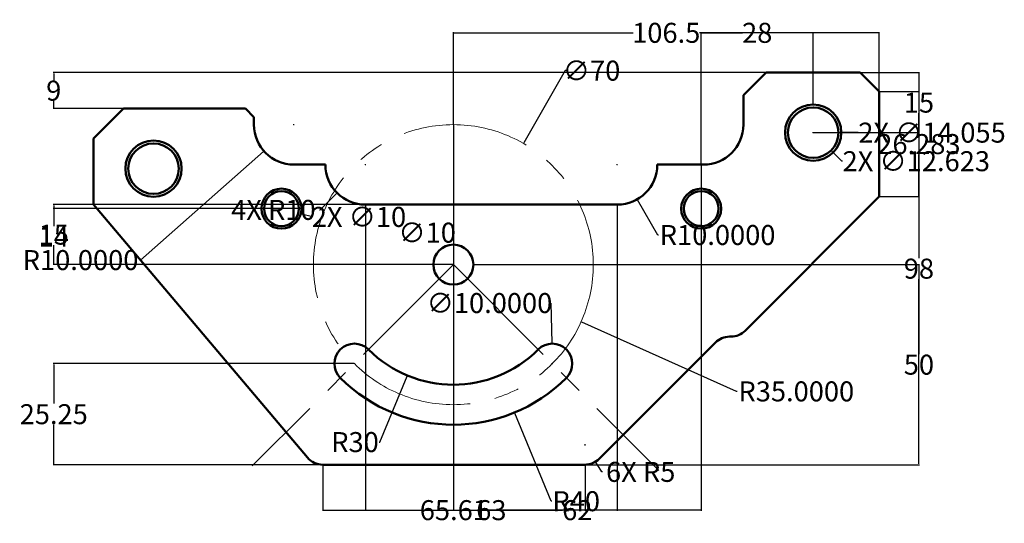
# Model space of a CAD drawing. Units: inches. Extents: x 2702 to 2948, y 1752 to 1878.
import ezdxf

# ---------------------------------------------------------------- set-up
doc = ezdxf.new("R2010")
doc.units = ezdxf.units.IN
doc.header["$MEASUREMENT"] = 0
doc.linetypes.add('CENTER', pattern=[50.8, 31.75, -6.35, 6.35, -6.35])
for name, color, linetype, lineweight in [('M-CNTR', 4, 'CENTER', 18), ('M-CONS', 8, 'Continuous', 13), ('M-DIMS', 2, 'Continuous', 25), ('M-OUTL', 7, 'Continuous', 50)]:
    doc.layers.add(name, color=color, linetype=linetype, lineweight=lineweight)
doc.styles.get("Standard").update_dxf_attribs({"font": 'arial.ttf'})
doc.dimstyles.get("Standard").update_dxf_attribs({"dimtxt": 5, "dimasz": 0.18, "dimexe": 0.18, "dimexo": 0.0625, "dimgap": 0.09, "dimtad": 0, "dimtih": 1, "dimtoh": 1, "dimdec": 4, "dimzin": 0, "dimdsep": 46, "dimtxsty": 'Standard', "dimcen": 0.09, "dimadec": 0, "dimazin": 0, "dimtfac": 1, "dimtdec": 4, "dimtofl": 0, "dimtmove": 0, "dimatfit": 3, "dimfxl": 1, "dimtolj": 1, "dimtzin": 0, "dimarcsym": 0})

# ---------------------------------------------------------------- blocks, each defined once
blk = doc.blocks.new('*D1')
at = {"layer": 'Defpoints', "color": 0, "transparency": 16777216}
for p in [(2851.5, 1841.74), (2856.48, 1833.07)]:
    blk.add_point(p, dxfattribs=at)
at = {"layer": 'M-DIMS', "color": 0, "lineweight": -2, "transparency": 16777216}
for p, q in [((2851.41, 1841.74), (2851.59, 1841.74)), ((2851.5, 1841.65), (2851.5, 1841.83)), ((2861.61, 1824.15), (2856.57, 1832.91)), ((2861.79, 1824.15), (2861.61, 1824.15))]:
    blk.add_line(p, q, dxfattribs=at)
at = {"layer": 'M-DIMS', "color": 0, "transparency": 16777216}
blk.add_solid([(2856.6, 1832.93), (2856.55, 1832.9), (2856.48, 1833.07)], dxfattribs=at)
at = {"layer": 'M-DIMS', "color": 0, "transparency": 16777216, "insert": (2876.59, 1824.15), "char_height": 5, "attachment_point": 5}
blk.add_mtext('\\A1;R10.0000', dxfattribs=at)
blk = doc.blocks.new('*D2')
at = {"layer": 'Defpoints', "color": 0, "transparency": 16777216}
for p in [(2770.62, 1851.74), (2763.12, 1845.12)]:
    blk.add_point(p, dxfattribs=at)
at = {"layer": 'M-DIMS', "color": 0, "lineweight": -2, "transparency": 16777216}
for p, q in [((2770.53, 1851.74), (2770.71, 1851.74)), ((2770.62, 1851.65), (2770.62, 1851.83)), ((2732.22, 1817.88), (2762.98, 1845.01)), ((2732.04, 1817.88), (2732.22, 1817.88))]:
    blk.add_line(p, q, dxfattribs=at)
at = {"layer": 'M-DIMS', "color": 0, "transparency": 16777216}
blk.add_solid([(2762.97, 1845.03), (2763, 1844.98), (2763.12, 1845.12)], dxfattribs=at)
at = {"layer": 'M-DIMS', "color": 0, "transparency": 16777216, "insert": (2717.25, 1817.88), "char_height": 5, "attachment_point": 5}
blk.add_mtext('\\A1;R10.0000', dxfattribs=at)
blk = doc.blocks.new('*D3')
at = {"layer": 'Defpoints', "color": 0, "transparency": 16777216}
for p in [(2810.5, 1816.74), (2842.45, 1802.45)]:
    blk.add_point(p, dxfattribs=at)
at = {"layer": 'M-DIMS', "color": 0, "lineweight": -2, "transparency": 16777216}
for p, q in [((2810.41, 1816.74), (2810.59, 1816.74)), ((2810.5, 1816.65), (2810.5, 1816.83)), ((2881.3, 1785.06), (2842.61, 1802.37)), ((2881.48, 1785.06), (2881.3, 1785.06))]:
    blk.add_line(p, q, dxfattribs=at)
at = {"layer": 'M-DIMS', "color": 0, "transparency": 16777216}
blk.add_solid([(2842.62, 1802.4), (2842.6, 1802.34), (2842.45, 1802.45)], dxfattribs=at)
at = {"layer": 'M-DIMS', "color": 0, "transparency": 16777216, "insert": (2896.28, 1785.06), "char_height": 5, "attachment_point": 5}
blk.add_mtext('\\A1;R35.0000', dxfattribs=at)
blk = doc.blocks.new('*D4')
at = {"layer": 'Defpoints', "color": 0, "transparency": 16777216}
for p in [(2835.11, 1796.99), (2835.38, 1786.99)]:
    blk.add_point(p, dxfattribs=at)
at = {"layer": 'M-DIMS', "color": 0, "lineweight": -2, "transparency": 16777216}
for p, q in [((2834.66, 1807.14), (2834.84, 1807.14)), ((2834.84, 1807.14), (2835.11, 1797.17)), ((2835.16, 1791.99), (2835.34, 1791.99)), ((2835.25, 1791.9), (2835.25, 1792.08))]:
    blk.add_line(p, q, dxfattribs=at)
at = {"layer": 'M-DIMS', "color": 0, "transparency": 16777216}
blk.add_solid([(2835.14, 1797.17), (2835.08, 1797.17), (2835.11, 1796.99)], dxfattribs=at)
at = {"layer": 'M-DIMS', "color": 0, "transparency": 16777216, "insert": (2819.53, 1807.14), "char_height": 5, "attachment_point": 5}
blk.add_mtext('\\A1;∅10.0000', dxfattribs=at)
blk = doc.blocks.new('MOUNT-HOLE-LARGE')
for radius in [7.03, 7.03, 7.03, 6.31]:
    blk.add_circle((0, 0), radius)
blk = doc.blocks.new('MOUNT-HOLE-SMALL')
for radius in [5, 4.36]:
    blk.add_circle((0, 0), radius)
blk = doc.blocks.new('*D7')
at = {"layer": 'Defpoints', "color": 0, "transparency": 16777216}
for p in [(2912.28, 1864.74), (2926.95, 1864.74), (2843.43, 1766.74)]:
    blk.add_point(p, dxfattribs=at)
at = {"layer": 'M-DIMS', "color": 0, "lineweight": -2, "transparency": 16777216}
for p, q in [((2912.35, 1864.74), (2927.13, 1864.74)), ((2926.95, 1864.56), (2926.95, 1818.38)), ((2926.95, 1766.92), (2926.95, 1813.1)), ((2843.49, 1766.74), (2927.13, 1766.74))]:
    blk.add_line(p, q, dxfattribs=at)
at = {"layer": 'M-DIMS', "color": 0, "transparency": 16777216}
for points in [[(2926.92, 1864.56), (2926.98, 1864.56), (2926.95, 1864.74)], [(2926.92, 1766.92), (2926.98, 1766.92), (2926.95, 1766.74)]]:
    blk.add_solid(points, dxfattribs=at)
at = {"layer": 'M-DIMS', "color": 0, "transparency": 16777216, "insert": (2926.95, 1815.74), "char_height": 5, "attachment_point": 5}
blk.add_mtext('\\A1;98', dxfattribs=at)
blk = doc.blocks.new('*D8')
at = {"layer": 'Defpoints', "color": 0, "transparency": 16777216}
for p in [(2917, 1874.69), (2917, 1860.02), (2810.5, 1851.74)]:
    blk.add_point(p, dxfattribs=at)
at = {"layer": 'M-DIMS', "color": 0, "lineweight": -2, "transparency": 16777216}
for p, q in [((2810.5, 1851.8), (2810.5, 1874.87)), ((2810.68, 1874.69), (2855.44, 1874.69)), ((2916.82, 1874.69), (2872.06, 1874.69)), ((2917, 1860.08), (2917, 1874.87))]:
    blk.add_line(p, q, dxfattribs=at)
at = {"layer": 'M-DIMS', "color": 0, "transparency": 16777216}
for points in [[(2810.68, 1874.72), (2810.68, 1874.66), (2810.5, 1874.69)], [(2916.82, 1874.72), (2916.82, 1874.66), (2917, 1874.69)]]:
    blk.add_solid(points, dxfattribs=at)
at = {"layer": 'M-DIMS', "color": 0, "transparency": 16777216, "insert": (2863.75, 1874.69), "char_height": 5, "attachment_point": 5}
blk.add_mtext('\\A1;106.5', dxfattribs=at)
blk = doc.blocks.new('*D9')
at = {"layer": 'Defpoints', "color": 0, "transparency": 16777216}
for p in [(2810.5, 1851.74), (2872.5, 1841.74), (2872.5, 1755.37)]:
    blk.add_point(p, dxfattribs=at)
at = {"layer": 'M-DIMS', "color": 0, "lineweight": -2, "transparency": 16777216}
for p, q in [((2810.5, 1851.68), (2810.5, 1755.19)), ((2872.5, 1841.68), (2872.5, 1755.19)), ((2810.68, 1755.37), (2837.84, 1755.37)), ((2872.32, 1755.37), (2845.16, 1755.37))]:
    blk.add_line(p, q, dxfattribs=at)
at = {"layer": 'M-DIMS', "color": 0, "transparency": 16777216}
for points in [[(2810.68, 1755.4), (2810.68, 1755.34), (2810.5, 1755.37)], [(2872.32, 1755.4), (2872.32, 1755.34), (2872.5, 1755.37)]]:
    blk.add_solid(points, dxfattribs=at)
at = {"layer": 'M-DIMS', "color": 0, "transparency": 16777216, "insert": (2841.5, 1755.37), "char_height": 5, "attachment_point": 5}
blk.add_mtext('\\A1;62', dxfattribs=at)
blk = doc.blocks.new('*D10')
at = {"layer": 'Defpoints', "color": 0, "transparency": 16777216}
for p in [(2900.5, 1874.69), (2900.5, 1856.77), (2872.5, 1841.74)]:
    blk.add_point(p, dxfattribs=at)
at = {"layer": 'M-DIMS', "color": 0, "lineweight": -2, "transparency": 16777216}
for p, q in [((2872.5, 1841.8), (2872.5, 1874.87)), ((2872.68, 1874.69), (2882.78, 1874.69)), ((2900.32, 1874.69), (2890.22, 1874.69)), ((2900.5, 1856.83), (2900.5, 1874.87))]:
    blk.add_line(p, q, dxfattribs=at)
at = {"layer": 'M-DIMS', "color": 0, "transparency": 16777216}
for points in [[(2872.68, 1874.72), (2872.68, 1874.66), (2872.5, 1874.69)], [(2900.32, 1874.72), (2900.32, 1874.66), (2900.5, 1874.69)]]:
    blk.add_solid(points, dxfattribs=at)
at = {"layer": 'M-DIMS', "color": 0, "transparency": 16777216, "insert": (2886.5, 1874.69), "char_height": 5, "attachment_point": 5}
blk.add_mtext('\\A1;28', dxfattribs=at)
blk = doc.blocks.new('*D11')
at = {"layer": 'Defpoints', "color": 0, "transparency": 16777216}
for p in [(2815.5, 1816.74), (2926.95, 1816.74), (2843.43, 1766.74)]:
    blk.add_point(p, dxfattribs=at)
at = {"layer": 'M-DIMS', "color": 0, "lineweight": -2, "transparency": 16777216}
for p, q in [((2815.56, 1816.74), (2927.13, 1816.74)), ((2926.95, 1816.56), (2926.95, 1794.38)), ((2926.95, 1766.92), (2926.95, 1789.1)), ((2843.49, 1766.74), (2927.13, 1766.74))]:
    blk.add_line(p, q, dxfattribs=at)
at = {"layer": 'M-DIMS', "color": 0, "transparency": 16777216}
for points in [[(2926.92, 1816.56), (2926.98, 1816.56), (2926.95, 1816.74)], [(2926.92, 1766.92), (2926.98, 1766.92), (2926.95, 1766.74)]]:
    blk.add_solid(points, dxfattribs=at)
at = {"layer": 'M-DIMS', "color": 0, "transparency": 16777216, "insert": (2926.95, 1791.74), "char_height": 5, "attachment_point": 5}
blk.add_mtext('\\A1;50', dxfattribs=at)
blk = doc.blocks.new('*D12')
at = {"layer": 'Defpoints', "color": 0, "transparency": 16777216}
for p in [(2710.55, 1830.74), (2772.5, 1830.74), (2805.5, 1816.74)]:
    blk.add_point(p, dxfattribs=at)
at = {"layer": 'M-DIMS', "color": 0, "lineweight": -2, "transparency": 16777216}
for p, q in [((2772.44, 1830.74), (2710.37, 1830.74)), ((2710.55, 1830.56), (2710.55, 1826.34)), ((2710.55, 1816.92), (2710.55, 1821.14)), ((2805.44, 1816.74), (2710.37, 1816.74))]:
    blk.add_line(p, q, dxfattribs=at)
at = {"layer": 'M-DIMS', "color": 0, "transparency": 16777216}
for points in [[(2710.52, 1830.56), (2710.58, 1830.56), (2710.55, 1830.74)], [(2710.52, 1816.92), (2710.58, 1816.92), (2710.55, 1816.74)]]:
    blk.add_solid(points, dxfattribs=at)
at = {"layer": 'M-DIMS', "color": 0, "transparency": 16777216, "insert": (2710.55, 1823.74), "char_height": 5, "attachment_point": 5}
blk.add_mtext('\\A1;14', dxfattribs=at)
blk = doc.blocks.new('*D13')
at = {"layer": 'Defpoints', "color": 0, "transparency": 16777216}
for p in [(2912.28, 1864.74), (2926.95, 1864.74), (2900.5, 1849.74)]:
    blk.add_point(p, dxfattribs=at)
at = {"layer": 'M-DIMS', "color": 0, "lineweight": -2, "transparency": 16777216}
for p, q in [((2912.35, 1864.74), (2927.13, 1864.74)), ((2926.95, 1864.56), (2926.95, 1859.88)), ((2926.95, 1849.92), (2926.95, 1854.6)), ((2900.56, 1849.74), (2927.13, 1849.74))]:
    blk.add_line(p, q, dxfattribs=at)
at = {"layer": 'M-DIMS', "color": 0, "transparency": 16777216}
for points in [[(2926.92, 1864.56), (2926.98, 1864.56), (2926.95, 1864.74)], [(2926.92, 1849.92), (2926.98, 1849.92), (2926.95, 1849.74)]]:
    blk.add_solid(points, dxfattribs=at)
at = {"layer": 'M-DIMS', "color": 0, "transparency": 16777216, "insert": (2926.95, 1857.24), "char_height": 5, "attachment_point": 5}
blk.add_mtext('\\A1;15', dxfattribs=at)
blk = doc.blocks.new('*D14')
at = {"layer": 'Defpoints', "color": 0, "transparency": 16777216}
for p in [(2788.5, 1831.74), (2851.5, 1831.74), (2851.5, 1755.37)]:
    blk.add_point(p, dxfattribs=at)
at = {"layer": 'M-DIMS', "color": 0, "lineweight": -2, "transparency": 16777216}
for p, q in [((2788.5, 1831.68), (2788.5, 1755.19)), ((2851.5, 1831.68), (2851.5, 1755.19)), ((2788.68, 1755.37), (2816.31, 1755.37)), ((2851.32, 1755.37), (2823.68, 1755.37))]:
    blk.add_line(p, q, dxfattribs=at)
at = {"layer": 'M-DIMS', "color": 0, "transparency": 16777216}
for points in [[(2788.68, 1755.4), (2788.68, 1755.34), (2788.5, 1755.37)], [(2851.32, 1755.4), (2851.32, 1755.34), (2851.5, 1755.37)]]:
    blk.add_solid(points, dxfattribs=at)
at = {"layer": 'M-DIMS', "color": 0, "transparency": 16777216, "insert": (2820, 1755.37), "char_height": 5, "attachment_point": 5}
blk.add_mtext('\\A1;63', dxfattribs=at)
blk = doc.blocks.new('*D15')
at = {"layer": 'Defpoints', "color": 0, "transparency": 16777216}
for p in [(2777.82, 1766.74), (2843.43, 1766.74), (2843.43, 1755.37)]:
    blk.add_point(p, dxfattribs=at)
at = {"layer": 'M-DIMS', "color": 0, "lineweight": -2, "transparency": 16777216}
for p, q in [((2777.82, 1766.68), (2777.82, 1755.19)), ((2843.43, 1766.68), (2843.43, 1755.19)), ((2778, 1755.37), (2802.57, 1755.37)), ((2843.25, 1755.37), (2818.68, 1755.37))]:
    blk.add_line(p, q, dxfattribs=at)
at = {"layer": 'M-DIMS', "color": 0, "transparency": 16777216}
for points in [[(2778, 1755.4), (2778, 1755.34), (2777.82, 1755.37)], [(2843.25, 1755.4), (2843.25, 1755.34), (2843.43, 1755.37)]]:
    blk.add_solid(points, dxfattribs=at)
at = {"layer": 'M-DIMS', "color": 0, "transparency": 16777216, "insert": (2810.62, 1755.37), "char_height": 5, "attachment_point": 5}
blk.add_mtext('\\A1;65.61', dxfattribs=at)
blk = doc.blocks.new('*D16')
at = {"layer": 'Defpoints', "color": 0, "transparency": 16777216}
for p in [(2788.5, 1831.74), (2710.55, 1816.74), (2810.5, 1816.74)]:
    blk.add_point(p, dxfattribs=at)
at = {"layer": 'M-DIMS', "color": 0, "lineweight": -2, "transparency": 16777216}
for p, q in [((2788.44, 1831.74), (2710.37, 1831.74)), ((2710.55, 1831.56), (2710.55, 1826.88)), ((2710.55, 1816.92), (2710.55, 1821.6)), ((2810.44, 1816.74), (2710.37, 1816.74))]:
    blk.add_line(p, q, dxfattribs=at)
at = {"layer": 'M-DIMS', "color": 0, "transparency": 16777216}
for points in [[(2710.52, 1831.56), (2710.58, 1831.56), (2710.55, 1831.74)], [(2710.52, 1816.92), (2710.58, 1816.92), (2710.55, 1816.74)]]:
    blk.add_solid(points, dxfattribs=at)
at = {"layer": 'M-DIMS', "color": 0, "transparency": 16777216, "insert": (2710.55, 1824.24), "char_height": 5, "attachment_point": 5}
blk.add_mtext('\\A1;15', dxfattribs=at)
blk = doc.blocks.new('*D17')
at = {"layer": 'Defpoints', "color": 0, "transparency": 16777216}
for p in [(2710.55, 1864.74), (2888.72, 1864.74), (2728, 1855.74)]:
    blk.add_point(p, dxfattribs=at)
at = {"layer": 'M-DIMS', "color": 0, "lineweight": -2, "transparency": 16777216}
for p, q in [((2888.65, 1864.74), (2710.37, 1864.74)), ((2710.55, 1864.56), (2710.55, 1862.88)), ((2710.55, 1855.92), (2710.55, 1857.6)), ((2727.94, 1855.74), (2710.37, 1855.74))]:
    blk.add_line(p, q, dxfattribs=at)
at = {"layer": 'M-DIMS', "color": 0, "transparency": 16777216}
for points in [[(2710.52, 1864.56), (2710.58, 1864.56), (2710.55, 1864.74)], [(2710.52, 1855.92), (2710.58, 1855.92), (2710.55, 1855.74)]]:
    blk.add_solid(points, dxfattribs=at)
at = {"layer": 'M-DIMS', "color": 0, "transparency": 16777216, "insert": (2710.55, 1860.24), "char_height": 5, "attachment_point": 5}
blk.add_mtext('\\A1;9', dxfattribs=at)
blk = doc.blocks.new('*D18')
at = {"layer": 'Defpoints', "color": 0, "transparency": 16777216}
for p in [(2917, 1860.02), (2926.95, 1860.02), (2917, 1833.74)]:
    blk.add_point(p, dxfattribs=at)
at = {"layer": 'M-DIMS', "color": 0, "lineweight": -2, "transparency": 16777216}
for p, q in [((2917.06, 1860.02), (2927.13, 1860.02)), ((2926.95, 1859.84), (2926.95, 1849.52)), ((2926.95, 1833.92), (2926.95, 1844.24)), ((2917.06, 1833.74), (2927.13, 1833.74))]:
    blk.add_line(p, q, dxfattribs=at)
at = {"layer": 'M-DIMS', "color": 0, "transparency": 16777216}
for points in [[(2926.92, 1859.84), (2926.98, 1859.84), (2926.95, 1860.02)], [(2926.92, 1833.92), (2926.98, 1833.92), (2926.95, 1833.74)]]:
    blk.add_solid(points, dxfattribs=at)
at = {"layer": 'M-DIMS', "color": 0, "transparency": 16777216, "insert": (2926.95, 1846.88), "char_height": 5, "attachment_point": 5}
blk.add_mtext('\\A1;26.283', dxfattribs=at)
blk = doc.blocks.new('*D19')
at = {"layer": 'Defpoints', "color": 0, "transparency": 16777216}
for p in [(2785.75, 1791.99), (2710.55, 1766.74), (2777.82, 1766.74)]:
    blk.add_point(p, dxfattribs=at)
at = {"layer": 'M-DIMS', "color": 0, "lineweight": -2, "transparency": 16777216}
for p, q in [((2785.69, 1791.99), (2710.37, 1791.99)), ((2710.55, 1791.81), (2710.55, 1782.01)), ((2710.55, 1766.92), (2710.55, 1776.72)), ((2777.76, 1766.74), (2710.37, 1766.74))]:
    blk.add_line(p, q, dxfattribs=at)
at = {"layer": 'M-DIMS', "color": 0, "transparency": 16777216}
for points in [[(2710.52, 1791.81), (2710.58, 1791.81), (2710.55, 1791.99)], [(2710.52, 1766.92), (2710.58, 1766.92), (2710.55, 1766.74)]]:
    blk.add_solid(points, dxfattribs=at)
at = {"layer": 'M-DIMS', "color": 0, "transparency": 16777216, "insert": (2710.55, 1779.36), "char_height": 5, "attachment_point": 5}
blk.add_mtext('\\A1;25.25', dxfattribs=at)
blk = doc.blocks.new('*D20')
at = {"layer": 'Defpoints', "color": 0, "transparency": 16777216}
for p in [(2810.5, 1816.74), (2825.8, 1779.78)]:
    blk.add_point(p, dxfattribs=at)
at = {"layer": 'M-DIMS', "color": 0, "lineweight": -2, "transparency": 16777216}
for p, q in [((2810.41, 1816.74), (2810.59, 1816.74)), ((2810.5, 1816.65), (2810.5, 1816.83)), ((2834.99, 1757.61), (2825.87, 1779.62)), ((2835.17, 1757.61), (2834.99, 1757.61))]:
    blk.add_line(p, q, dxfattribs=at)
at = {"layer": 'M-DIMS', "color": 0, "transparency": 16777216}
blk.add_solid([(2825.9, 1779.63), (2825.85, 1779.6), (2825.8, 1779.78)], dxfattribs=at)
at = {"layer": 'M-DIMS', "color": 0, "transparency": 16777216, "insert": (2841.22, 1757.61), "char_height": 5, "attachment_point": 5}
blk.add_mtext('\\A1;R40', dxfattribs=at)
blk = doc.blocks.new('*D21')
at = {"layer": 'Defpoints', "color": 0, "transparency": 16777216}
for p in [(2810.5, 1816.74), (2799.02, 1789.02)]:
    blk.add_point(p, dxfattribs=at)
at = {"layer": 'M-DIMS', "color": 0, "lineweight": -2, "transparency": 16777216}
for p, q in [((2810.41, 1816.74), (2810.59, 1816.74)), ((2810.5, 1816.65), (2810.5, 1816.83)), ((2792.13, 1772.39), (2798.95, 1788.86)), ((2791.95, 1772.39), (2792.13, 1772.39))]:
    blk.add_line(p, q, dxfattribs=at)
at = {"layer": 'M-DIMS', "color": 0, "transparency": 16777216}
blk.add_solid([(2798.92, 1788.87), (2798.98, 1788.84), (2799.02, 1789.02)], dxfattribs=at)
at = {"layer": 'M-DIMS', "color": 0, "transparency": 16777216, "insert": (2785.9, 1772.39), "char_height": 5, "attachment_point": 5}
blk.add_mtext('\\A1;R30', dxfattribs=at)
blk = doc.blocks.new('*D22')
at = {"layer": 'Defpoints', "color": 0, "transparency": 16777216}
for p in [(2843.43, 1771.74), (2846.07, 1767.49)]:
    blk.add_point(p, dxfattribs=at)
at = {"layer": 'M-DIMS', "color": 0, "lineweight": -2, "transparency": 16777216}
for p, q in [((2843.34, 1771.74), (2843.52, 1771.74)), ((2843.43, 1771.65), (2843.43, 1771.83)), ((2847.65, 1764.94), (2846.16, 1767.34)), ((2847.83, 1764.94), (2847.65, 1764.94))]:
    blk.add_line(p, q, dxfattribs=at)
at = {"layer": 'M-DIMS', "color": 0, "transparency": 16777216}
blk.add_solid([(2846.19, 1767.35), (2846.14, 1767.32), (2846.07, 1767.49)], dxfattribs=at)
at = {"layer": 'M-DIMS', "color": 0, "transparency": 16777216, "insert": (2857.36, 1764.94), "char_height": 5, "attachment_point": 5}
blk.add_mtext('\\A1;6X R5', dxfattribs=at)
blk = doc.blocks.new('*D23')
at = {"layer": 'Defpoints', "color": 0, "transparency": 16777216}
for p in [(2893.47, 1849.74), (2907.53, 1849.74)]:
    blk.add_point(p, dxfattribs=at)
at = {"layer": 'M-DIMS', "color": 0, "lineweight": -2, "transparency": 16777216}
for p, q in [((2900.41, 1849.74), (2900.59, 1849.74)), ((2900.5, 1849.65), (2900.5, 1849.83)), ((2911.74, 1849.74), (2907.71, 1849.74))]:
    blk.add_line(p, q, dxfattribs=at)
at = {"layer": 'M-DIMS', "color": 0, "transparency": 16777216}
blk.add_solid([(2907.71, 1849.77), (2907.71, 1849.71), (2907.53, 1849.74)], dxfattribs=at)
at = {"layer": 'M-DIMS', "color": 0, "transparency": 16777216, "insert": (2930.23, 1849.74), "char_height": 5, "attachment_point": 5}
blk.add_mtext('\\A1;2X ∅14.055', dxfattribs=at)
blk = doc.blocks.new('*D24')
at = {"layer": 'Defpoints', "color": 0, "transparency": 16777216}
for p in [(2896.04, 1854.2), (2904.96, 1845.28)]:
    blk.add_point(p, dxfattribs=at)
at = {"layer": 'M-DIMS', "color": 0, "lineweight": -2, "transparency": 16777216}
for p, q in [((2900.41, 1849.74), (2900.59, 1849.74)), ((2900.5, 1849.65), (2900.5, 1849.83)), ((2907.64, 1842.6), (2905.09, 1845.15)), ((2907.82, 1842.6), (2907.64, 1842.6))]:
    blk.add_line(p, q, dxfattribs=at)
at = {"layer": 'M-DIMS', "color": 0, "transparency": 16777216}
blk.add_solid([(2905.11, 1845.17), (2905.07, 1845.13), (2904.96, 1845.28)], dxfattribs=at)
at = {"layer": 'M-DIMS', "color": 0, "transparency": 16777216, "insert": (2926.29, 1842.6), "char_height": 5, "attachment_point": 5}
blk.add_mtext('\\A1;2X ∅12.623', dxfattribs=at)
blk = doc.blocks.new('*D25')
at = {"layer": 'Defpoints', "color": 0, "transparency": 16777216}
for p in [(2810.5, 1821.74), (2810.5, 1811.74)]:
    blk.add_point(p, dxfattribs=at)
at = {"layer": 'M-DIMS', "color": 0, "lineweight": -2, "transparency": 16777216}
for p, q in [((2810.32, 1824.74), (2810.5, 1824.74)), ((2810.5, 1824.74), (2810.5, 1821.92)), ((2810.41, 1816.74), (2810.59, 1816.74)), ((2810.5, 1816.65), (2810.5, 1816.83))]:
    blk.add_line(p, q, dxfattribs=at)
at = {"layer": 'M-DIMS', "color": 0, "transparency": 16777216}
blk.add_solid([(2810.53, 1821.92), (2810.47, 1821.92), (2810.5, 1821.74)], dxfattribs=at)
at = {"layer": 'M-DIMS', "color": 0, "transparency": 16777216, "insert": (2803.94, 1824.74), "char_height": 5, "attachment_point": 5}
blk.add_mtext('\\A1;∅10', dxfattribs=at)
blk = doc.blocks.new('*D26')
at = {"layer": 'Defpoints', "color": 0, "transparency": 16777216}
for p in [(2762.67, 1832.03), (2772.33, 1829.45)]:
    blk.add_point(p, dxfattribs=at)
at = {"layer": 'M-DIMS', "color": 0, "lineweight": -2, "transparency": 16777216}
for p, q in [((2767.41, 1830.74), (2767.59, 1830.74)), ((2767.5, 1830.65), (2767.5, 1830.83)), ((2775.23, 1828.67), (2772.5, 1829.4))]:
    blk.add_line(p, q, dxfattribs=at)
at = {"layer": 'M-DIMS', "color": 0, "transparency": 16777216}
blk.add_solid([(2772.51, 1829.43), (2772.5, 1829.37), (2772.33, 1829.45)], dxfattribs=at)
at = {"layer": 'M-DIMS', "color": 0, "transparency": 16777216, "insert": (2786.89, 1828.67), "char_height": 5, "attachment_point": 5}
blk.add_mtext('\\A1;2X ∅10', dxfattribs=at)
blk = doc.blocks.new('*D27')
at = {"layer": 'Defpoints', "color": 0, "transparency": 16777216}
for p in [(2788.5, 1841.74), (2781.43, 1834.67)]:
    blk.add_point(p, dxfattribs=at)
at = {"layer": 'M-DIMS', "color": 0, "lineweight": -2, "transparency": 16777216}
for p, q in [((2788.41, 1841.74), (2788.59, 1841.74)), ((2788.5, 1841.65), (2788.5, 1841.83)), ((2777.19, 1830.43), (2781.3, 1834.54)), ((2777.01, 1830.43), (2777.19, 1830.43))]:
    blk.add_line(p, q, dxfattribs=at)
at = {"layer": 'M-DIMS', "color": 0, "transparency": 16777216}
blk.add_solid([(2781.28, 1834.56), (2781.32, 1834.52), (2781.43, 1834.67)], dxfattribs=at)
at = {"layer": 'M-DIMS', "color": 0, "transparency": 16777216, "insert": (2765.48, 1830.43), "char_height": 5, "attachment_point": 5}
blk.add_mtext('\\A1;4X R10', dxfattribs=at)
blk = doc.blocks.new('*D28')
at = {"layer": 'Defpoints', "color": 0, "transparency": 16777216}
for p in [(2828, 1847.05), (2793, 1786.43)]:
    blk.add_point(p, dxfattribs=at)
at = {"layer": 'M-DIMS', "color": 0, "lineweight": -2, "transparency": 16777216}
for p, q in [((2838.5, 1865.24), (2828.09, 1847.21)), ((2838.68, 1865.24), (2838.5, 1865.24)), ((2810.41, 1816.74), (2810.59, 1816.74)), ((2810.5, 1816.65), (2810.5, 1816.83))]:
    blk.add_line(p, q, dxfattribs=at)
at = {"layer": 'M-DIMS', "color": 0, "transparency": 16777216}
blk.add_solid([(2828.06, 1847.22), (2828.12, 1847.19), (2828, 1847.05)], dxfattribs=at)
at = {"layer": 'M-DIMS', "color": 0, "transparency": 16777216, "insert": (2845.06, 1865.24), "char_height": 5, "attachment_point": 5}
blk.add_mtext('\\A1;∅70', dxfattribs=at)

msp = doc.modelspace()

# ---------------------------------------------------------------- linework, layer by layer
at = {"layer": 'M-CNTR'}
for q in [(2760.21471, 1766.45406), (2861.92048, 1765.31737)]:
    msp.add_line((2810.49925, 1816.73861), q, dxfattribs=at)
msp.add_circle((2810.49925, 1816.73861), 35, dxfattribs=at)
at = {"layer": 'M-CONS'}
msp.add_line((2872.49925, 1841.73861), (2872.49925, 1830.73861), dxfattribs=at)
at = {"layer": 'M-OUTL'}
for p, q in [((2888.71585, 1864.73861), (2883.05899, 1859.08175)), ((2900.49925, 1864.73861), (2888.71585, 1864.73861)), ((2900.49925, 1864.73861), (2912.28266, 1864.73861)), ((2912.28266, 1864.73861), (2916.99925, 1860.02201)), ((2916.99925, 1860.02201), (2916.99925, 1833.73861)), ((2883.05899, 1859.08175), (2883.05899, 1851.73861)), ((2727.99925, 1855.73861), (2720.49925, 1848.23861)), ((2727.99925, 1855.73861), (2758.49925, 1855.73861)), ((2758.49925, 1855.73861), (2760.62057, 1853.61729)), ((2760.62057, 1853.61729), (2760.62057, 1851.73861)), ((2720.49925, 1831.73861), (2720.49925, 1848.23861)), ((2778.49925, 1841.73861), (2770.62057, 1841.73861)), ((2861.49925, 1841.73861), (2872.49925, 1841.73861)), ((2873.05899, 1841.73861), (2872.49925, 1841.73861)), ((2916.99925, 1833.73861), (2883.46372, 1800.20307)), ((2774.00131, 1768.50889), (2720.49925, 1831.73861)), ((2810.49925, 1831.73861), (2788.49925, 1831.73861)), ((2810.49925, 1831.73861), (2851.49925, 1831.73861)), ((2879.57032, 1798.73861), (2879.92818, 1798.73861)), ((2846.96372, 1768.20307), (2876.03479, 1797.27414)), ((2777.81825, 1766.73861), (2843.42818, 1766.73861))]:
    msp.add_line(p, q, dxfattribs=at)
msp.add_circle((2810.49925, 1816.73861), 5, dxfattribs=at)
for centre, radius, start, end in [((2770.62057, 1851.73861), 10, 180, 270), ((2873.05899, 1851.73861), 10, 270, 0), ((2788.49925, 1841.73861), 10, 180, 270), ((2851.49925, 1841.73861), 10, 270, 0), ((2879.57032, 1793.73861), 5, 90, 135), ((2879.92818, 1803.73861), 5, 270, 315), ((2785.75051, 1791.98987), 5, 45, 225), ((2810.49925, 1816.73861), 30, 225, 315), ((2835.24799, 1791.98987), 5, 315, 135), ((2810.49925, 1816.73861), 40, 225, 315), ((2777.81825, 1771.73861), 5, 220.2363583, 270), ((2843.42818, 1771.73861), 5, 270, 315)]:
    msp.add_arc(centre, radius, start, end, dxfattribs=at)

# ---------------------------------------------------------------- block references
for name, p in [('MOUNT-HOLE-LARGE', (2900.49925, 1849.73861)), ('MOUNT-HOLE-LARGE', (2735.49925, 1840.73861)), ('MOUNT-HOLE-SMALL', (2767.49925, 1830.73861)), ('MOUNT-HOLE-SMALL', (2872.49925, 1830.73861))]:
    msp.add_blockref(name, p, dxfattribs=at)

# ---------------------------------------------------------------- dimensions: what is measured, and where the dimension line sits
at = {"layer": 'M-DIMS'}
for base, p1, p2, override, picture, middle in [((2916.99925, 1874.68861), (2810.49925, 1851.73861), (2916.99925, 1860.02201), {"dimdec": 1, "dimlfac": 1, "dimrnd": 0, "dimzin": 0, "dimdsep": 46, "dimlunit": 2}, '*D8', (2863.74925, 1874.68861)), ((2900.49925, 1874.68861), (2872.49925, 1841.73861), (2900.49925, 1856.76616), {"dimdec": 0, "dimlfac": 1, "dimrnd": 0, "dimzin": 0, "dimdsep": 46, "dimlunit": 2}, '*D10', (2886.49925, 1874.68861)), ((2872.49925, 1755.36737), (2810.49925, 1851.73861), (2872.49925, 1841.73861), {"dimdec": 0, "dimlfac": 1, "dimrnd": 0, "dimzin": 0, "dimdsep": 46, "dimlunit": 2}, '*D9', (2841.49925, 1755.36737)), ((2851.49925, 1755.36737), (2788.49925, 1831.73861), (2851.49925, 1831.73861), {"dimdec": 0, "dimlfac": 1, "dimrnd": 0, "dimzin": 0, "dimdsep": 46, "dimlunit": 2}, '*D14', (2819.99925, 1755.36737)), ((2843.42818, 1755.36737), (2777.81825, 1766.73861), (2843.42818, 1766.73861), {"dimdec": 2, "dimlfac": 1, "dimrnd": 0, "dimzin": 0, "dimdsep": 46, "dimlunit": 2}, '*D15', (2810.62322, 1755.36737))]:
    dim = msp.add_linear_dim(base=base, p1=p1, p2=p2, dimstyle='Standard', override=override, dxfattribs=at)
    dim.commit()
    dim.dimension.update_dxf_attribs({"geometry": picture, "text_midpoint": middle})
for p1, p2, override, picture, middle in [((2792.99923, 1786.42773), (2827.99928, 1847.04948), {"dimdec": 0, "dimlfac": 1, "dimrnd": 0, "dimzin": 0, "dimdsep": 46, "dimlunit": 2}, '*D28', (2845.06193, 1865.236)), ((2810.4995, 1811.73861), (2810.499, 1821.73861), {"dimdec": 0, "dimlfac": 1, "dimrnd": 0, "dimzin": 0, "dimdsep": 46, "dimlunit": 2}, '*D25', (2803.93622, 1824.73861)), ((2835.38378, 1786.99171), (2835.11219, 1796.98802), {"dimclrd": 0, "dimclre": 0, "dimclrt": 0}, '*D4', (2819.53393, 1807.14169))]:
    dim = msp.add_diameter_dim_2p(p1=p1, p2=p2, dimstyle='Standard', override=override, dxfattribs=at)
    dim.commit()
    dim.dimension.update_dxf_attribs({"geometry": picture, "text_midpoint": middle, "dimtype": 163})
for base, p1, p2, override, picture, middle in [((2710.54925, 1864.73861), (2727.99925, 1855.73861), (2888.71585, 1864.73861), {"dimdec": 0, "dimlfac": 1, "dimrnd": 0, "dimzin": 0, "dimdsep": 46, "dimlunit": 2}, '*D17', (2710.54925, 1860.23861)), ((2926.94925, 1864.73861), (2843.42818, 1766.73861), (2912.28265, 1864.73861), {"dimdec": 0, "dimlfac": 1, "dimrnd": 0, "dimzin": 0, "dimdsep": 46, "dimlunit": 2}, '*D7', (2926.94925, 1815.73861)), ((2926.94925, 1864.73861), (2900.49925, 1849.73861), (2912.28265, 1864.73861), {"dimdec": 0, "dimlfac": 1, "dimrnd": 0, "dimzin": 0, "dimdsep": 46, "dimlunit": 2}, '*D13', (2926.94925, 1857.23861)), ((2926.94925, 1860.02201), (2916.99925, 1833.73861), (2916.99925, 1860.02201), {"dimdec": 3, "dimlfac": 1, "dimrnd": 0, "dimzin": 0, "dimdsep": 46, "dimlunit": 2}, '*D18', (2926.94925, 1846.88031)), ((2710.54925, 1816.73861), (2788.49925, 1831.73861), (2810.49925, 1816.73861), {"dimdec": 0, "dimlfac": 1, "dimrnd": 0, "dimzin": 0, "dimdsep": 46, "dimlunit": 2}, '*D16', (2710.54925, 1824.23861)), ((2710.54925, 1830.73861), (2805.49925, 1816.73861), (2772.49925, 1830.73861), {"dimdec": 0, "dimlfac": 1, "dimrnd": 0, "dimzin": 0, "dimdsep": 46, "dimlunit": 2}, '*D12', (2710.54925, 1823.73861)), ((2926.94925, 1816.73861), (2843.42818, 1766.73861), (2815.49925, 1816.73861), {"dimdec": 0, "dimlfac": 1, "dimrnd": 0, "dimzin": 0, "dimdsep": 46, "dimlunit": 2}, '*D11', (2926.94925, 1791.73861)), ((2710.54925, 1766.73861), (2785.75051, 1791.98987), (2777.81825, 1766.73861), {"dimdec": 2, "dimlfac": 1, "dimrnd": 0, "dimzin": 0, "dimdsep": 46, "dimlunit": 2}, '*D19', (2710.54925, 1779.36424))]:
    dim = msp.add_linear_dim(base=base, p1=p1, p2=p2, angle=90, dimstyle='Standard', override=override, dxfattribs=at)
    dim.commit()
    dim.dimension.update_dxf_attribs({"geometry": picture, "text_midpoint": middle})
for p1, p2, override, picture, middle in [((2893.4717, 1849.73721), (2907.5268, 1849.74), {"dimdec": 3, "dimlfac": 1, "dimrnd": 0, "dimzin": 0, "dimdsep": 46, "dimlunit": 2}, '*D23', (2911.74333, 1849.74084)), ((2896.03543, 1854.20028), (2904.96308, 1845.27693), {"dimdec": 3, "dimlfac": 1, "dimrnd": 0, "dimzin": 0, "dimdsep": 46, "dimlunit": 2}, '*D24', (2926.29131, 1842.59992)), ((2762.66943, 1832.03196), (2772.32908, 1829.44525), {"dimdec": 0, "dimlfac": 1, "dimrnd": 0, "dimzin": 0, "dimdsep": 46, "dimlunit": 2}, '*D26', (2775.22697, 1828.66923))]:
    dim = msp.add_diameter_dim_2p(p1=p1, p2=p2, text='2X <>', dimstyle='Standard', override=override, dxfattribs=at)
    dim.commit()
    dim.dimension.update_dxf_attribs({"geometry": picture, "text_midpoint": middle, "dimtype": 163})
for center, mpoint, override, picture, middle in [((2770.62057, 1851.73861), (2763.11996, 1845.12492), {"dimclrd": 0, "dimclre": 0, "dimclrt": 0}, '*D2', (2717.24892, 1817.88221)), ((2851.49925, 1841.73861), (2856.48404, 1833.06959), {"dimclrd": 0, "dimclre": 0, "dimclrt": 0}, '*D1', (2876.58968, 1824.14687)), ((2810.49925, 1816.73861), (2799.01869, 1789.02225), {"dimdec": 0, "dimlfac": 1, "dimrnd": 0, "dimzin": 0, "dimdsep": 46, "dimlunit": 2}, '*D21', (2785.89514, 1772.39243)), ((2810.49925, 1816.73861), (2842.44791, 1802.44584), {"dimclrd": 0, "dimclre": 0, "dimclrt": 0}, '*D3', (2896.27536, 1785.06454)), ((2810.49925, 1816.73861), (2825.80488, 1779.78272), {"dimdec": 0, "dimlfac": 1, "dimrnd": 0, "dimzin": 0, "dimdsep": 46, "dimlunit": 2}, '*D20', (2841.22346, 1757.60918))]:
    dim = msp.add_radius_dim(center=center, mpoint=mpoint, dimstyle='Standard', override=override, dxfattribs=at)
    dim.commit()
    dim.dimension.update_dxf_attribs({"geometry": picture, "text_midpoint": middle, "dimtype": 164})
for center, mpoint, text, picture, middle in [((2788.49925, 1841.73861), (2781.42786, 1834.66786), '4X <>', '*D27', (2765.47744, 1830.42541)), ((2843.42818, 1771.73861), (2846.06724, 1767.4918), '6X <>', '*D22', (2857.35621, 1764.94371))]:
    dim = msp.add_radius_dim(center=center, mpoint=mpoint, text=text, dimstyle='Standard', override={"dimdec": 0, "dimlfac": 1, "dimrnd": 0, "dimzin": 0, "dimdsep": 46, "dimlunit": 2}, dxfattribs=at)
    dim.commit()
    dim.dimension.update_dxf_attribs({"geometry": picture, "text_midpoint": middle, "dimtype": 164})

doc.saveas('drawing.dxf')
